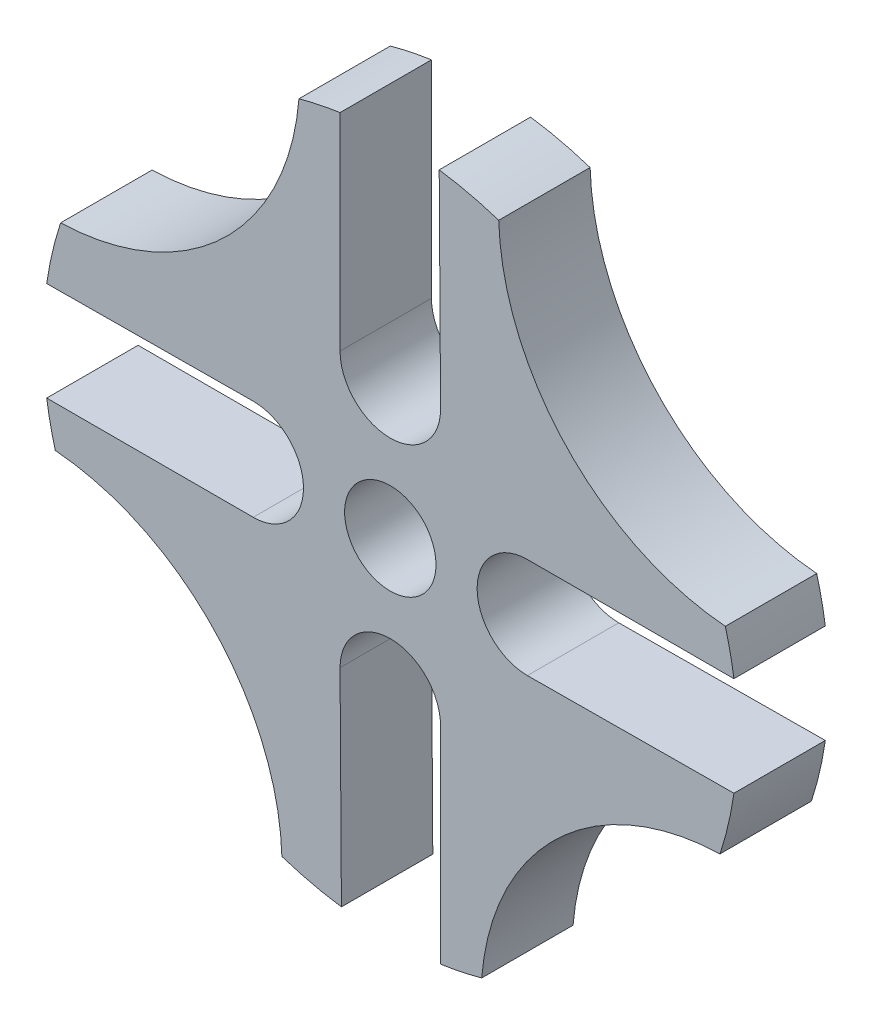
SolidWorks part; units mm, degrees
material "Plain Carbon Steel"
ref_plane "Front Plane" through (0, 0, 0) normal (0, 0, 1) x (1, 0, 0)
ref_plane "Top Plane" through (0, 0, 0) normal (0, 1, 0) x (1, 0, 0)
ref_plane "Right Plane" through (0, 0, 0) normal (1, 0, 0) x (0, 0, -1)
sketch "Geneva Wheel Profile" plane through (0, 0, 0) normal (0, 0, 1) x (1, 0, 0)
  line L0 (0, 43.1118) -> (0, -52.5025) construction
  line L1 (-57.3686, 0) -> (53.6123, 0) construction
  line L2 (0, 15) -> (0, 61.0998) construction
  line L3 (-5.5, 15) -> (-5.5, 37.5999)
  line L4 (5.5, 15) -> (5.3501, 37.6)
  line L5 (15, 5.5) -> (37.5999, 5.5)
  line L6 (15, -5.5) -> (37.6, -5.3501)
  line L7 (5.5, -15) -> (5.5, -37.5999)
  line L8 (-5.5, -15) -> (-5.3501, -37.6)
  line L9 (-15, -5.5) -> (-37.5999, -5.5)
  line L10 (-15, 5.5) -> (-37.6, 5.3501)
  line L11 (-10, 2.2913) -> (-10, -2.2913)
  line L12 (10, 2.2913) -> (10, -2.2913)
  line L14 (10, 43.1118) -> (10, -52.5025) construction
  line L15 (-10, 43.1118) -> (-10, -52.5025) construction
  circle A0 centre (0, 0) radius 5
  arc A1 (-5.5, 37.5999) -> (-10, 36.6606) centre (0, 0) ccw
  arc A2 (-5.5, 15) -> (5.5, 15) centre (0, 15) ccw
  arc A4 (15, 5.5) -> (15, -5.5) centre (15, 0) ccw
  arc A5 (5.5, -15) -> (-5.5, -15) centre (0, -15) ccw
  arc A6 (-15, -5.5) -> (-15, 5.5) centre (-15, 0) ccw
  arc A8 (11.8627, 36.0785) -> (5.3501, 37.6) centre (0, 0) ccw
  arc A10 (37.5999, 5.5) -> (36.6606, 10) centre (0, 0) ccw
  arc A11 (36.0785, -11.8627) -> (37.6, -5.3501) centre (0, 0) ccw
  arc A12 (5.5, -37.5999) -> (10, -36.6606) centre (0, 0) ccw
  arc A13 (-11.8627, -36.0785) -> (-5.3501, -37.6) centre (0, 0) ccw
  arc A14 (-37.5999, -5.5) -> (-36.6606, -10) centre (0, 0) ccw
  arc A15 (-36.0785, 11.8627) -> (-37.6, 5.3501) centre (0, 0) ccw
  arc A16 (11.8627, 36.0785) -> (36.6606, 10) centre (38.8499, 36.9111) ccw
  arc A17 (36.0785, -11.8627) -> (10, -36.6606) centre (36.9111, -38.8499) ccw
  arc A18 (-11.8627, -36.0785) -> (-36.6606, -10) centre (-38.8499, -36.9111) ccw
  arc A19 (-36.0785, 11.8627) -> (-10, 36.6606) centre (-36.9111, 38.8499) ccw
  point P10 (0, 38.0499)
  point P32 (0, 0)
  point P55 (0, 0)
  point P60 (0, 0)
  dimension "D1" = 76
  dimension "D2" = 10
  dimension "D4" = 5.5
  dimension "D9" = 27
  dimension "D3" = 15
  dimension "D10" = 5.3501
  dimension "D11" = 37.6
  dimension "D13" = 38.8499
  dimension "D14" = 36.9111
  dimension "D15" = 46.0998
  dimension "D6" = 10
  dimension "D7" = 10
  dimension "D5" = 4
  dimension "D8" = 4
  dimension "D12" = 4
extrude "Geneva Wheel Body 10mm" add sketch "Geneva Wheel Profile" along normal blind 10 contours A19 A15 L10 A6 L9 A14 A18 A13 L8 A5 L7 A12 A17 A11 L6 A4 L5 A10 A16 A8 L4 A2 L3 A1 A0
